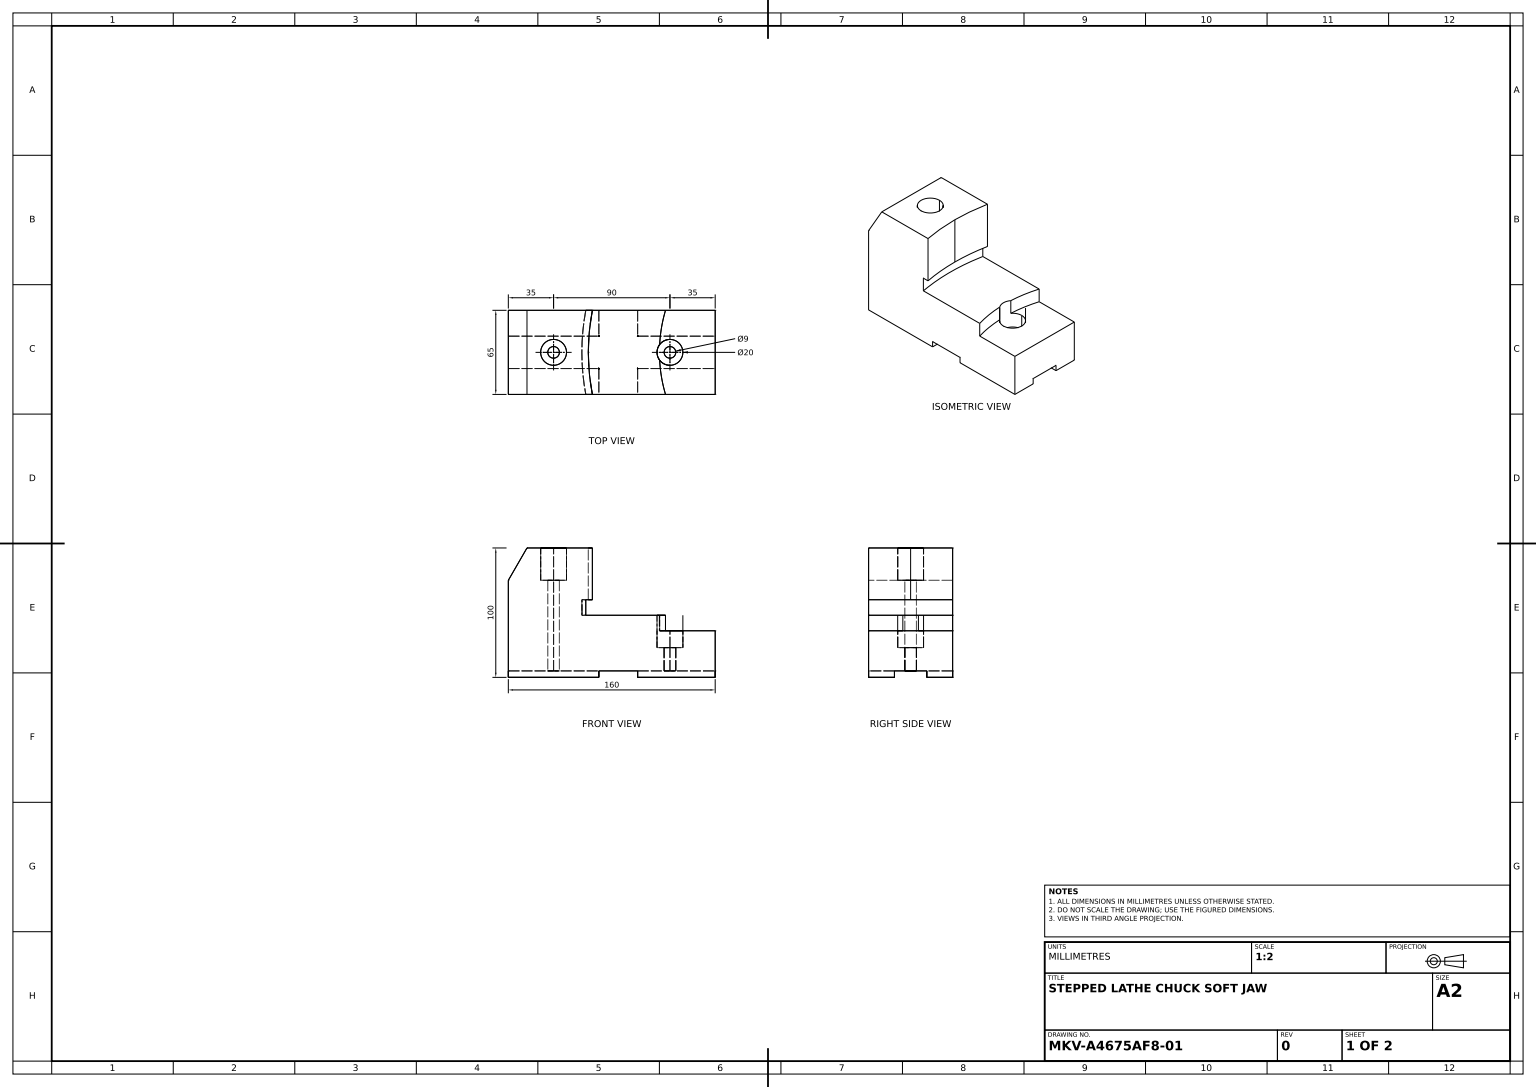
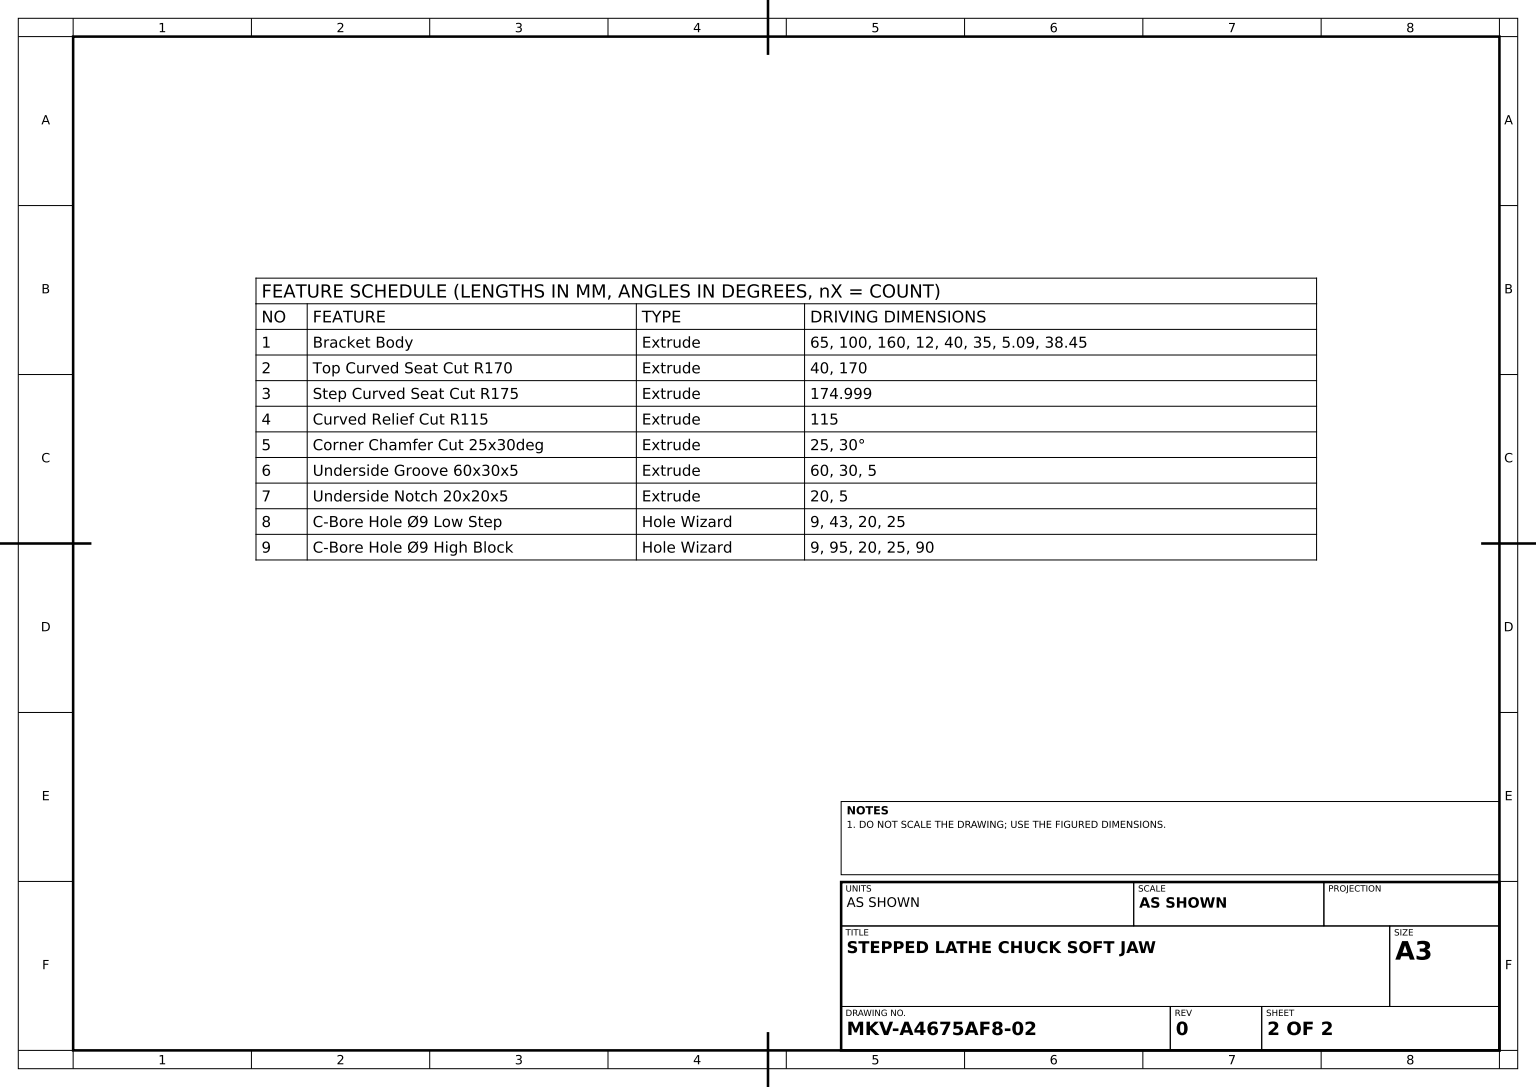
SolidWorks part; units mm, degrees
material "Plain Carbon Steel"
ref_plane "Front Plane" through (0, 0, 0) normal (0, 0, 1) x (1, 0, 0)
ref_plane "Top Plane" through (0, 0, 0) normal (0, 1, 0) x (1, 0, 0)
ref_plane "Right Plane" through (0, 0, 0) normal (1, 0, 0) x (0, 0, -1)
sketch "Bracket Side Profile Sketch" plane through (0, 0, 0) normal (0, 0, 1) x (1, 0, 0)
  line L0 (35, 0) -> (-125, 0)
  line L1 (-125, 0) -> (-125, 100)
  line L2 (-125, 100) -> (-60, 100)
  line L4 (-65.09, 48) -> (-3.45, 48)
  line L5 (-3.45, 48) -> (-3.45, 36)
  line L6 (-3.45, 36) -> (35, 36)
  line L7 (35, 36) -> (35, 0)
  line L8 (-60, 100) -> (-60, 60)
  line L9 (-60, 60) -> (-65.09, 60)
  line L10 (-65.09, 60) -> (-65.09, 48)
  dimension "D1" = 100
  dimension "D2" = 160
  dimension "D3" = 40
  dimension "D4" = 12
  dimension "D5" = 12
  dimension "D6" = 65
  dimension "D7" = 35
  dimension "D8" = 5.09
  dimension "D9" = 38.45
extrude "Bracket Body" add sketch "Bracket Side Profile Sketch" along normal mid plane 65
sketch "Top Curved Seat Sketch R170" plane through (0, 100, 0) normal (0, 1, 0) x (1, 0, 0)
  arc A0 (-60, 32.5) -> (-60, -32.5) centre (106.8645, 0) ccw
  line M5 (-60, -32.5) -> (-60, 32.5)
  dimension "D1" = 170
extrude "Top Curved Seat Cut R170" cut sketch "Top Curved Seat Sketch R170" against normal blind 40 and the other way through all contours A0 M5
sketch "Step Curved Seat Sketch R175" plane through (0, 48, 0) normal (0, 1, 0) x (1, 0, 0)
  line L0 (-65.09, -32.5) -> (-65.09, 32.5) construction
  line L1 (-65.09, -32.5) -> (-65.09, 32.5)
  arc A0 (-65.09, 32.5) -> (-65.09, -32.5) centre (106.8645, 0) ccw
  line M2 (-65.09, 32.5) -> (-65.09, -32.5)
  dimension "D1" = 174.9988
extrude "Step Curved Seat Cut R175" cut sketch "Step Curved Seat Sketch R175" along normal up to surface (12 mm away) contours A0 M2
sketch "Curved Relief Sketch R115" plane through (0, 36, 0) normal (0, 1, 0) x (1, 0, 0)
  line L1 (-3.45, -32.5) -> (-3.45, 32.5) construction
  line L2 (-3.45, -32.5) -> (-3.45, 32.5)
  arc A0 (-3.45, -32.5) -> (-3.45, 32.5) centre (106.8621, 0) cw
  dimension "D1" = 115
extrude "Curved Relief Cut R115" cut sketch "Curved Relief Sketch R115" along normal up to surface (12 mm away) contours A0 L2 up to face at (-35.0311, 48, 0)
sketch "Corner Chamfer Sketch 25x30deg" plane through (0, 0, 32.5) normal (0, 0, 1) x (1, 0, 0)
  line L0 (-125, 100) -> (-110.5662, 100)
  line L1 (-60, 100) -> (-125, 100) construction
  line L2 (-110.5662, 100) -> (-125, 75)
  line L3 (-125, 100) -> (-125, 0) construction
  line L4 (-125, 75) -> (-125, 100)
  dimension "D1" = 25
  dimension "D2" = 30
extrude "Corner Chamfer Cut 25x30deg" cut sketch "Corner Chamfer Sketch 25x30deg" against normal through all
sketch "Underside Groove Sketch 60x30" plane through (0, 0, 32.5) normal (0, 0, 1) x (1, 0, 0)
  line L0 (-125, 0) -> (35, 0) construction
  line L1 (-55, 0) -> (-25, 0)
  line L2 (-55, 0) -> (-55, 5)
  line L3 (-55, 5) -> (-25, 5)
  line L4 (-25, 0) -> (-25, 5)
  line L5 (35, 0) -> (35, 36) construction
  dimension "D1" = 60
  dimension "D2" = 30
  dimension "D3" = 5
extrude "Underside Groove 60x30x5" cut sketch "Underside Groove Sketch 60x30" against normal through all
sketch "Underside Notch Sketch 20x20" plane through (35, 0, 0) normal (1, 0, 0) x (0, 0, -1)
  line L0 (-32.5, 0) -> (32.5, 0) construction
  line L1 (-12.5, 0) -> (12.5, 0)
  line L2 (-12.5, 0) -> (-12.5, 5)
  line L3 (-12.5, 5) -> (12.5, 5)
  line L4 (12.5, 0) -> (12.5, 5)
  line L5 (-32.5, 0) -> (-32.5, 36) construction
  dimension "D1" = 20
  dimension "D2" = 20
  dimension "D3" = 5
extrude "Underside Notch 20x20x5" cut sketch "Underside Notch Sketch 20x20" against normal through all
hole_wizard "C-Bore Hole Ø9 Low Step" positions "Sketch11" profile "Sketch12" legacy end condition up to next
sketch "Sketch11" plane through (0, 48, 0) normal (0, 1, 0) x (1, 0, 0)
  point P0 (0, 0)
sketch "Sketch12" plane through (0, 48, 0) normal (1, 0, 0) x (0, 0, 1)
  line L0 (0, 0) -> (0, 43)
  line L1 (0, 43) -> (4.5, 43)
  line L2 (4.5, 43) -> (4.5, 25)
  line L3 (4.5, 25) -> (10, 25)
  line L4 (10, 25) -> (10, 0)
  line L5 (10, 0) -> (0, 0)
  line L6 (0, 110) -> (0, -10) construction
  dimension "Diameter" = 9
  dimension "Depth" = 43
  dimension "C-Bore Diameter" = 20
  dimension "C-Bore Depth" = 25
hole_wizard "C-Bore Hole Ø9 High Block" positions "Sketch13" profile "Sketch14" legacy end condition up to next
sketch "Sketch13" plane through (0, 100, 0) normal (0, 1, 0) x (1, 0, 0)
  point P0 (-90, 0)
  dimension "D1" = 90
sketch "Sketch14" plane through (-90, 100, 0) normal (1, 0, 0) x (0, 0, 1)
  line L0 (0, 0) -> (0, 95)
  line L1 (0, 95) -> (4.5, 95)
  line L2 (4.5, 95) -> (4.5, 25)
  line L3 (4.5, 25) -> (10, 25)
  line L4 (10, 25) -> (10, 0)
  line L5 (10, 0) -> (0, 0)
  line L6 (0, 110) -> (0, -10) construction
  dimension "Diameter" = 9
  dimension "Depth" = 95
  dimension "C-Bore Diameter" = 20
  dimension "C-Bore Depth" = 25
